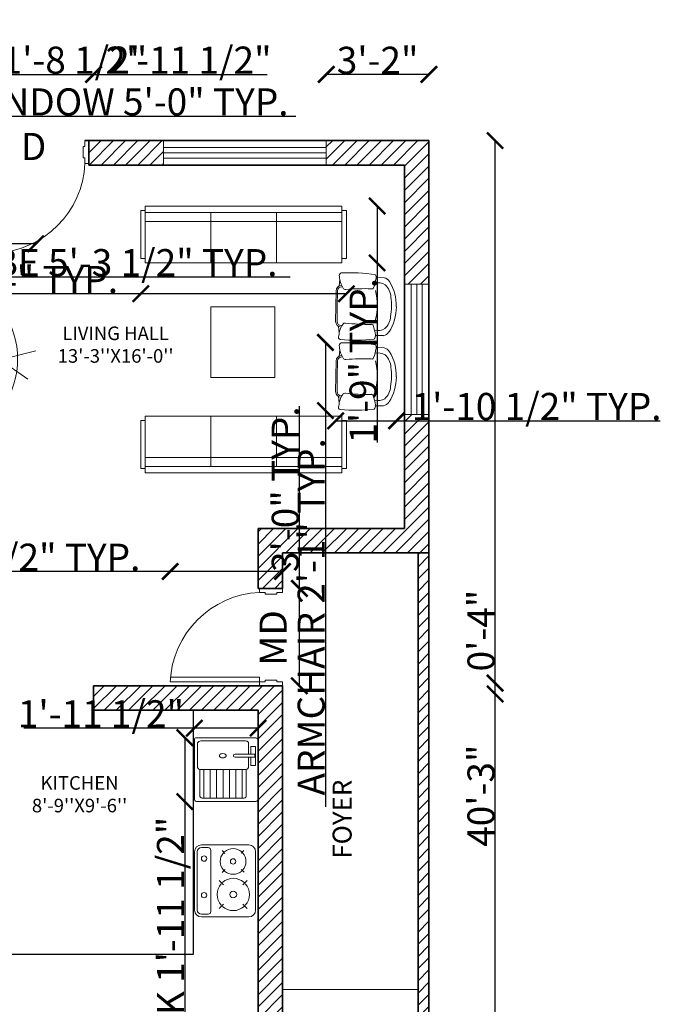
# Model space of a CAD drawing. Units: inches. Extents: x 1957 to 2456, y 1504 to 2088.
# Tile 6 of 6: x 2220 to 2456, y 1703 to 2066. Entities that reach past the tile are written whole.
import ezdxf

# ---------------------------------------------------------------- set-up
doc = ezdxf.new("R2010")
doc.units = ezdxf.units.IN
doc.header["$LTSCALE"] = 2
for name, color, linetype, lineweight in [('A-ANNO-DIMS', 2, 'Continuous', 18), ('A-ANNO-TEXT', 7, 'Continuous', 18), ('A-AREA-IDEN', 7, 'Continuous', 18), ('A-EQPM', 8, 'Continuous', 18), ('A-FLOR-FIXT', 8, 'Continuous', 18), ('A-FURN', 8, 'Continuous', 18), ('A-WALL-PATT', 8, 'Continuous', 13), ('Doors', 42, 'Continuous', 18), ('Kitchen', 60, 'Continuous', 25), ('Steps', 50, 'Continuous', 18), ('Walls', 7, 'Continuous', 35), ('Windows', 140, 'Continuous', 18)]:
    doc.layers.add(name, color=color, linetype=linetype, lineweight=lineweight)
doc.styles.get("Standard").update_dxf_attribs({"font": 'arial.ttf'})
doc.dimstyles.get("Standard").update_dxf_attribs({"dimtxt": 10, "dimasz": 6, "dimexe": 0.18, "dimexo": 0.0625, "dimgap": 0.09, "dimtad": 1, "dimdec": 1, "dimzin": 0, "dimdsep": 46, "dimlunit": 4, "dimtxsty": 'Standard', "dimblk": 'ARCHTICK', "dimcen": 0.09, "dimse1": 1, "dimse2": 1, "dimadec": 0, "dimazin": 0, "dimtfac": 1, "dimtdec": 1, "dimtofl": 0, "dimtmove": 0, "dimatfit": 3, "dimfxl": 1, "dimtolj": 1, "dimtzin": 0, "dimarcsym": 0})

# ---------------------------------------------------------------- blocks, each defined once
blk = doc.blocks.new('S_SINK12')
for p, q in [((0.25, 0.45), (0.25, 0)), ((0.35, 0.45), (0.35, 0)), ((0.45, 0.45), (0.45, 0)), ((0.55, 0.45), (0.55, 0)), ((0.65, 0.45), (0.65, 0)), ((0.75, 0.45), (0.75, 0)), ((0.85, 0.45), (0.85, 0))]:
    blk.add_line(p, q)
for points in [[(0, -0.469), (0, 0.469, -0.310961), (0.05, 0.5), (0.95, 0.5, -0.310466), (1, 0.469), (1, -0.469, -0.414214), (0.969, -0.5), (0.05, -0.5, -0.309971)], [(0.052, -0.195), (0.052, -0.242), (0.362, -0.242, 1), (0.362, -0.195)], [(0.5, -0.217), (0.503, -0.229, 0.107136), (0.516, -0.241, 0.076468), (0.534, -0.249), (0.554, -0.251), (0.575, -0.248, 0.076468), (0.592, -0.241, 0.107136), (0.604, -0.229), (0.608, -0.217), (0.604, -0.205, 0.107136), (0.592, -0.193, 0.076468), (0.575, -0.186), (0.554, -0.183), (0.532, -0.186, 0.076468), (0.516, -0.193, 0.107136), (0.503, -0.205)]]:
    blk.add_lwpolyline(points, format="xyb", close=True)
for points in [[(0.185, -0.001), (0.185, 0.419, -0.310466), (0.235, 0.45), (0.862, 0.45, -0.310466), (0.912, 0.419), (0.912, 0, -0.310466)], [(0.15, -0.195), (0.15, -0.031, -0.310466), (0.2, 0), (0.9, 0, -0.310466), (0.95, -0.031), (0.95, -0.419, -0.310466), (0.9, -0.45), (0.2, -0.45), (0.18, -0.448, -0.071009), (0.165, -0.442, -0.106323), (0.153, -0.432), (0.15, -0.422), (0.151, -0.419)]]:
    blk.add_lwpolyline(points, format="xyb")
for points in [[(0.114, -0.242), (0.114, -0.364), (0.039, -0.364), (0.039, -0.064), (0.114, -0.064), (0.114, -0.195)], [(0.15, -0.419), (0.15, -0.242)]]:
    blk.add_lwpolyline(points)
blk = doc.blocks.new('12PCOU09')
at = {"color": 0, "linetype": 'ByBlock'}
for p, q in [((26, 15), (3, 15)), ((26, -15), (3, -15))]:
    blk.add_line(p, q, dxfattribs=at)
for points in [[(2, 45), (2, 47), (24, 47), (24, 45)], [(2, -47), (2, -45), (24, -45), (24, -47)]]:
    blk.add_lwpolyline(points, close=True, dxfattribs=at)
for points in [[(2, -45), (0, -45), (0, 45), (2, 45)], [(3, -45), (3, 45)], [(7, 45), (7, -45)], [(24, 45), (26, 45), (26, -45), (24, -45)]]:
    blk.add_lwpolyline(points, dxfattribs=at)
blk = doc.blocks.new('banghe81')
for p, q in [((-500, 3000), (0, 3000)), ((-500, 2312), (-500, 3000)), ((0, 3000), (0, 0)), ((-925, 1843), (-450, 1517)), ((-607, 1930), (-419, 1930)), ((-607, 1117), (-607, 1930)), ((-419, 1930), (-419, 1117)), ((-107, 1742), (-419, 1867)), ((-107, 1305), (-107, 1742)), ((-450, 1517), (-1057, 1361)), ((-482, 1617), (-482, 1430)), ((-419, 1617), (-482, 1617)), ((-482, 1430), (-419, 1430)), ((-419, 1180), (-107, 1305)), ((-419, 1117), (-607, 1117)), ((-500, 0), (-500, 688)), ((0, 0), (-500, 0)), ((-500, 0), (-500, 0))]:
    blk.add_line(p, q)
blk.add_arc((695, 1500), 1445, 145.7945, 214.2055)
blk = doc.blocks.new('A$C198557BC')
for p, q in [((-0.412, 0.581), (-0.41, 0.695)), ((0.425, 0.571), (0.425, 0.685)), ((-0.291, 0.046), (-0.382, 0.055)), ((-0.299, 0.083), (-0.299, 0.085)), ((0, 0.02), (-0.22, 0.023)), ((0, 0), (-0.22, 0.003)), ((0, 0.02), (0.221, 0.017)), ((0, 0), (0.22, -0.003)), ((0.291, 0.039), (0.383, 0.046)), ((0.301, 0.077), (0.301, 0.078))]:
    blk.add_line(p, q)
for centre, radius, start, end in [((-0.003, 0.196), 0.675, 88.9141, 121.2698), ((0.005, 0.189), 0.683, 57.6049, 89.6023), ((-0.288, 0.668), 0.124, 121.5636, 167.5307), ((-0.132, 0.606), 0.205, 148.9368, 191.7767), ((-0.109, 0.514), 0.28, 94.1154, 135.1368), ((-0.012, 0.135), 0.669, 87.9714, 100.088), ((-0.041, -0.271), 1.076, 79.8996, 87.1923), ((0.131, 0.526), 0.263, 42.8435, 86.2186), ((0.304, 0.661), 0.124, 11.1649, 57.132), ((1.987, 0.194), 2.469, 171.2505, 182.7738), ((-0.42, 0.533), 0.0491, 69.3538, 131.4415), ((-0.498, -0.067), 0.653, 68.9876, 81.6584), ((-0.015, -0.198), 0.795, 73.9397, 105.2329), ((0.496, -0.078), 0.653, 97.0372, 109.708), ((0.146, 0.603), 0.205, 346.9189, 29.7588), ((0.427, 0.504), 0.0668, 46.1176, 99.1612), ((-0.269, 0.522), 0.0208, 332.4461, 75.1743), ((3.087, 0.412), 3.339, 178.2785, 184.601), ((-3.076, 0.483), 3.339, 354.0946, 0.4171), ((0.281, 0.516), 0.0208, 103.5213, 206.2495), ((-1.903, 0.273), 2.393, 354.9918, 6.6966), ((-0.281, 0.139), 0.0403, 300.8178, 7.8066), ((-0.444, 0.084), 0.0362, 194.4565, 300.6699), ((-0.452, 0.425), 0.374, 274.1336, 300.8386), ((-0.219, 0.083), 0.08, 179.3478, 269.3478), ((-0.219, 0.083), 0.06, 179.3478, 269.3478), ((0.221, 0.077), 0.08, 269.3478, 359.3478), ((0.221, 0.077), 0.06, 269.3478, 359.3478), ((0.284, 0.133), 0.0403, 170.889, 237.8778), ((0.462, 0.415), 0.374, 237.857, 264.562), ((0.446, 0.074), 0.0362, 238.0257, 344.2391)]:
    blk.add_arc(centre, radius, start, end)
blk = doc.blocks.new('AP0B05')
for p, q in [((35, 100), (35, 880)), ((75, 100), (75, 878.9))]:
    blk.add_line(p, q)
for points in [[(0, 100), (0, -100), (35, -100), (35, -50), (50, -50), (50, 50), (35, 50), (35, 100)], [(850, 100), (850, -100), (815, -100), (815, -50), (800, -50), (800, 50), (815, 50), (815, 100)]]:
    blk.add_lwpolyline(points, close=True)
blk.add_lwpolyline([(35, 100), (75, 100)])
blk.add_arc((-2.4, 62.6), 818.3, 2.62122, 87.37878)
blk = doc.blocks.new('WIN-48IN')
for p, q in [((0, 6.5), (48, 6.5)), ((0, 4.5), (48, 4.5)), ((0, 2.5), (48, 2.5))]:
    blk.add_line(p, q)
blk.add_lwpolyline([(0, 9), (48, 9), (48, 0), (0, 0)], close=True)
blk = doc.blocks.new('WIN-60IN')
for p, q in [((0, 6.5), (60, 6.5)), ((0, 4.5), (60, 4.5)), ((0, 2.5), (60, 2.5))]:
    blk.add_line(p, q)
blk.add_lwpolyline([(0, 9), (60, 9), (60, 0), (0, 0)], close=True)
blk = doc.blocks.new('_ArchTick')
at = {"color": 0, "linetype": 'ByBlock', "const_width": 0.15}
blk.add_lwpolyline([(-0.5, -0.5), (0.5, 0.5)], dxfattribs=at)
blk = doc.blocks.new('*D19')
at = {"layer": 'A-ANNO-DIMS', "color": 0, "lineweight": -2, "transparency": 16777216}
for p, q in [((2275.61, 1862.36), (2088.68, 1862.36)), ((2317.03, 1862.36), (2275.61, 1862.36))]:
    blk.add_line(p, q, dxfattribs=at)
at = {"layer": 'Defpoints', "color": 0, "transparency": 16777216}
for p in [(2275.61, 1862.36), (2275.61, 1856.15), (2317.03, 1856.15)]:
    blk.add_point(p, dxfattribs=at)
at = {"layer": 'A-ANNO-DIMS', "color": 0, "lineweight": -2, "transparency": 16777216, "xscale": 6, "yscale": 6, "zscale": 6, "rotation": 180}
blk.add_blockref('_ArchTick', (2275.61, 1862.36), dxfattribs=at)
at = {"layer": 'A-ANNO-DIMS', "color": 0, "lineweight": -2, "transparency": 16777216, "xscale": 6, "yscale": 6, "zscale": 6}
blk.add_blockref('_ArchTick', (2317.03, 1862.36), dxfattribs=at)
at = {"layer": 'A-ANNO-DIMS', "color": 0, "transparency": 16777216, "insert": (2179.14, 1867.63), "char_height": 10, "attachment_point": 5}
blk.add_mtext('\\A1;ENTRY DOOR 3\'-5 1/2" TYP.', dxfattribs=at)
blk = doc.blocks.new('*D20')
at = {"layer": 'A-ANNO-DIMS', "color": 0, "lineweight": -2, "transparency": 16777216}
for p, q in [((2323.25, 1856.15), (2323.25, 1923.28)), ((2323.25, 1820.22), (2323.25, 1856.15))]:
    blk.add_line(p, q, dxfattribs=at)
at = {"layer": 'Defpoints', "color": 0, "transparency": 16777216}
for p in [(2317.03, 1856.15), (2323.25, 1856.15), (2317.03, 1820.22)]:
    blk.add_point(p, dxfattribs=at)
at = {"layer": 'A-ANNO-DIMS', "color": 0, "lineweight": -2, "transparency": 16777216, "xscale": 6, "yscale": 6, "zscale": 6}
for p, rotation in [((2323.25, 1856.15), 90), ((2323.25, 1820.22), 270)]:
    blk.add_blockref('_ArchTick', p, dxfattribs=dict(at, rotation=rotation))
at = {"layer": 'A-ANNO-DIMS', "color": 0, "transparency": 16777216, "insert": (2318.05, 1892.71), "char_height": 10, "attachment_point": 5, "rotation": 90}
blk.add_mtext('\\A1;3\'-0" TYP.', dxfattribs=at)
blk = doc.blocks.new('*D25')
at = {"layer": 'A-ANNO-DIMS', "color": 0, "lineweight": -2, "transparency": 16777216}
for p, q in [((2129.18, 2030.22), (2189.18, 2030.22)), ((2189.18, 2030.22), (2321.9, 2030.22))]:
    blk.add_line(p, q, dxfattribs=at)
at = {"layer": 'Defpoints', "color": 0, "transparency": 16777216}
for p in [(2189.18, 2030.22), (2129.18, 2021.22), (2189.18, 2021.22)]:
    blk.add_point(p, dxfattribs=at)
at = {"layer": 'A-ANNO-DIMS', "color": 0, "lineweight": -2, "transparency": 16777216, "xscale": 6, "yscale": 6, "zscale": 6, "rotation": 180}
blk.add_blockref('_ArchTick', (2129.18, 2030.22), dxfattribs=at)
at = {"layer": 'A-ANNO-DIMS', "color": 0, "lineweight": -2, "transparency": 16777216, "xscale": 6, "yscale": 6, "zscale": 6}
blk.add_blockref('_ArchTick', (2189.18, 2030.22), dxfattribs=at)
at = {"layer": 'A-ANNO-DIMS', "color": 0, "transparency": 16777216, "insert": (2258.54, 2035.48), "char_height": 10, "attachment_point": 5}
blk.add_mtext('\\A1;WINDOW 5\'-0" TYP.', dxfattribs=at)
blk = doc.blocks.new('*D31')
at = {"layer": 'A-ANNO-DIMS', "color": 0, "lineweight": -2, "transparency": 16777216}
for p, q in [((2079.36, 1970.96), (2142.81, 1970.96)), ((2142.81, 1970.96), (2319.81, 1970.96))]:
    blk.add_line(p, q, dxfattribs=at)
at = {"layer": 'Defpoints', "color": 0, "transparency": 16777216}
for p in [(2079.36, 1980.47), (2142.81, 1980.47), (2142.81, 1970.96)]:
    blk.add_point(p, dxfattribs=at)
at = {"layer": 'A-ANNO-DIMS', "color": 0, "lineweight": -2, "transparency": 16777216, "xscale": 6, "yscale": 6, "zscale": 6, "rotation": 180}
blk.add_blockref('_ArchTick', (2079.36, 1970.96), dxfattribs=at)
at = {"layer": 'A-ANNO-DIMS', "color": 0, "lineweight": -2, "transparency": 16777216, "xscale": 6, "yscale": 6, "zscale": 6}
blk.add_blockref('_ArchTick', (2142.81, 1970.96), dxfattribs=at)
at = {"layer": 'A-ANNO-DIMS', "color": 0, "transparency": 16777216, "insert": (2234.31, 1976.22), "char_height": 10, "attachment_point": 5}
blk.add_mtext('\\A1;WARDROBE 5\'-3 1/2" TYP.', dxfattribs=at)
blk = doc.blocks.new('*D35')
at = {"layer": 'A-ANNO-DIMS', "color": 0, "lineweight": -2, "transparency": 16777216}
for p, q in [((2264.8, 1964.77), (2155.8, 1964.77)), ((2340.57, 1964.77), (2264.8, 1964.77))]:
    blk.add_line(p, q, dxfattribs=at)
at = {"layer": 'Defpoints', "color": 0, "transparency": 16777216}
for p in [(2264.8, 1976.14), (2340.57, 1976.14), (2264.8, 1964.77)]:
    blk.add_point(p, dxfattribs=at)
at = {"layer": 'A-ANNO-DIMS', "color": 0, "lineweight": -2, "transparency": 16777216, "xscale": 6, "yscale": 6, "zscale": 6, "rotation": 180}
blk.add_blockref('_ArchTick', (2264.8, 1964.77), dxfattribs=at)
at = {"layer": 'A-ANNO-DIMS', "color": 0, "lineweight": -2, "transparency": 16777216, "xscale": 6, "yscale": 6, "zscale": 6}
blk.add_blockref('_ArchTick', (2340.57, 1964.77), dxfattribs=at)
at = {"layer": 'A-ANNO-DIMS', "color": 0, "transparency": 16777216, "insert": (2207.3, 1970.03), "char_height": 10, "attachment_point": 5}
blk.add_mtext('\\A1;SOFA 6\'-4" TYP.', dxfattribs=at)
blk = doc.blocks.new('*D36')
at = {"layer": 'A-ANNO-DIMS', "color": 0, "lineweight": -2, "transparency": 16777216}
for p, q in [((2351.93, 1997.09), (2351.93, 1976.14)), ((2351.93, 1976.14), (2351.93, 1909.94))]:
    blk.add_line(p, q, dxfattribs=at)
at = {"layer": 'Defpoints', "color": 0, "transparency": 16777216}
for p in [(2340.57, 1997.09), (2340.57, 1976.14), (2351.93, 1976.14)]:
    blk.add_point(p, dxfattribs=at)
at = {"layer": 'A-ANNO-DIMS', "color": 0, "lineweight": -2, "transparency": 16777216, "xscale": 6, "yscale": 6, "zscale": 6}
for p, rotation in [((2351.93, 1997.09), 90), ((2351.93, 1976.14), 270)]:
    blk.add_blockref('_ArchTick', p, dxfattribs=dict(at, rotation=rotation))
at = {"layer": 'A-ANNO-DIMS', "color": 0, "transparency": 16777216, "insert": (2346.74, 1940.04), "char_height": 10, "attachment_point": 5, "rotation": 90}
blk.add_mtext('\\A1;1\'-9" TYP.', dxfattribs=at)
blk = doc.blocks.new('*D37')
at = {"layer": 'A-ANNO-DIMS', "color": 0, "lineweight": -2, "transparency": 16777216}
for p, q in [((2332.87, 1946.81), (2332.87, 1921.7)), ((2332.87, 1921.7), (2332.87, 1775.6))]:
    blk.add_line(p, q, dxfattribs=at)
at = {"layer": 'Defpoints', "color": 0, "transparency": 16777216}
for p in [(2336.64, 1946.81), (2332.87, 1921.7), (2336.64, 1921.7)]:
    blk.add_point(p, dxfattribs=at)
at = {"layer": 'A-ANNO-DIMS', "color": 0, "lineweight": -2, "transparency": 16777216, "xscale": 6, "yscale": 6, "zscale": 6}
for p, rotation in [((2332.87, 1946.81), 90), ((2332.87, 1921.7), 270)]:
    blk.add_blockref('_ArchTick', p, dxfattribs=dict(at, rotation=rotation))
at = {"layer": 'A-ANNO-DIMS', "color": 0, "transparency": 16777216, "insert": (2327.61, 1845.65), "char_height": 10, "attachment_point": 5, "rotation": 90}
blk.add_mtext('\\A1;ARMCHAIR 2\'-1" TYP.', dxfattribs=at)
blk = doc.blocks.new('*D38')
at = {"layer": 'A-ANNO-DIMS', "color": 0, "lineweight": -2, "transparency": 16777216}
for p, q in [((2336.64, 1917.93), (2359.07, 1917.93)), ((2359.07, 1917.93), (2456.34, 1917.93))]:
    blk.add_line(p, q, dxfattribs=at)
at = {"layer": 'Defpoints', "color": 0, "transparency": 16777216}
for p in [(2336.64, 1921.7), (2359.07, 1921.7), (2359.07, 1917.93)]:
    blk.add_point(p, dxfattribs=at)
at = {"layer": 'A-ANNO-DIMS', "color": 0, "lineweight": -2, "transparency": 16777216, "xscale": 6, "yscale": 6, "zscale": 6, "rotation": 180}
blk.add_blockref('_ArchTick', (2336.64, 1917.93), dxfattribs=at)
at = {"layer": 'A-ANNO-DIMS', "color": 0, "lineweight": -2, "transparency": 16777216, "xscale": 6, "yscale": 6, "zscale": 6}
blk.add_blockref('_ArchTick', (2359.07, 1917.93), dxfattribs=at)
at = {"layer": 'A-ANNO-DIMS', "color": 0, "transparency": 16777216, "insert": (2410.71, 1923.2), "char_height": 10, "attachment_point": 5}
blk.add_mtext('\\A1;1\'-10 1/2" TYP.', dxfattribs=at)
blk = doc.blocks.new('*D40')
at = {"layer": 'A-ANNO-DIMS', "color": 0, "lineweight": -2, "transparency": 16777216}
for p, q in [((2203.03, 1983.16), (2163.44, 1983.16)), ((2226.04, 1983.16), (2203.03, 1983.16))]:
    blk.add_line(p, q, dxfattribs=at)
at = {"layer": 'Defpoints', "color": 0, "transparency": 16777216}
for p in [(2203.03, 1983.16), (2203.03, 1973.36), (2226.04, 1973.36)]:
    blk.add_point(p, dxfattribs=at)
at = {"layer": 'A-ANNO-DIMS', "color": 0, "lineweight": -2, "transparency": 16777216, "xscale": 6, "yscale": 6, "zscale": 6, "rotation": 180}
blk.add_blockref('_ArchTick', (2203.03, 1983.16), dxfattribs=at)
at = {"layer": 'A-ANNO-DIMS', "color": 0, "lineweight": -2, "transparency": 16777216, "xscale": 6, "yscale": 6, "zscale": 6}
blk.add_blockref('_ArchTick', (2226.04, 1983.16), dxfattribs=at)
at = {"layer": 'A-ANNO-DIMS', "color": 0, "transparency": 16777216, "insert": (2180.24, 1988.27), "char_height": 10, "attachment_point": 5}
blk.add_mtext('\\A1;1\'-11"', dxfattribs=at)
blk = doc.blocks.new('*D41')
at = {"layer": 'A-ANNO-DIMS', "color": 0, "lineweight": -2, "transparency": 16777216}
for p, q in [((2281, 1801.1), (2281, 1777.56)), ((2281, 1777.56), (2281, 1677.29))]:
    blk.add_line(p, q, dxfattribs=at)
at = {"layer": 'Defpoints', "color": 0, "transparency": 16777216}
for p in [(2284.53, 1801.1), (2281, 1777.56), (2284.53, 1777.56)]:
    blk.add_point(p, dxfattribs=at)
at = {"layer": 'A-ANNO-DIMS', "color": 0, "lineweight": -2, "transparency": 16777216, "xscale": 6, "yscale": 6, "zscale": 6}
for p, rotation in [((2281, 1801.1), 90), ((2281, 1777.56), 270)]:
    blk.add_blockref('_ArchTick', p, dxfattribs=dict(at, rotation=rotation))
at = {"layer": 'A-ANNO-DIMS', "color": 0, "transparency": 16777216, "insert": (2275.74, 1724.42), "char_height": 10, "attachment_point": 5, "rotation": 90}
blk.add_mtext('\\A1;SINK 1\'-11 1/2"', dxfattribs=at)
blk = doc.blocks.new('*D42')
at = {"layer": 'A-ANNO-DIMS', "color": 0, "lineweight": -2, "transparency": 16777216}
for p, q in [((2284.53, 1804.64), (2221.64, 1804.64)), ((2308.03, 1804.64), (2284.53, 1804.64))]:
    blk.add_line(p, q, dxfattribs=at)
at = {"layer": 'Defpoints', "color": 0, "transparency": 16777216}
for p in [(2284.53, 1804.64), (2284.53, 1801.1), (2308.03, 1801.1)]:
    blk.add_point(p, dxfattribs=at)
at = {"layer": 'A-ANNO-DIMS', "color": 0, "lineweight": -2, "transparency": 16777216, "xscale": 6, "yscale": 6, "zscale": 6, "rotation": 180}
blk.add_blockref('_ArchTick', (2284.53, 1804.64), dxfattribs=at)
at = {"layer": 'A-ANNO-DIMS', "color": 0, "lineweight": -2, "transparency": 16777216, "xscale": 6, "yscale": 6, "zscale": 6}
blk.add_blockref('_ArchTick', (2308.03, 1804.64), dxfattribs=at)
at = {"layer": 'A-ANNO-DIMS', "color": 0, "transparency": 16777216, "insert": (2250.09, 1809.9), "char_height": 10, "attachment_point": 5}
blk.add_mtext('\\A1;1\'-11 1/2"', dxfattribs=at)
blk = doc.blocks.new('*D46')
at = {"layer": 'A-ANNO-DIMS', "color": 0, "lineweight": -2, "transparency": 16777216}
blk.add_line((2395.43, 1538.22), (2395.43, 2021.22), dxfattribs=at)
at = {"layer": 'Defpoints', "color": 0, "transparency": 16777216}
for p in [(2371.03, 2021.22), (2395.43, 2021.22), (2371.03, 1538.22)]:
    blk.add_point(p, dxfattribs=at)
at = {"layer": 'A-ANNO-DIMS', "color": 0, "lineweight": -2, "transparency": 16777216, "xscale": 6, "yscale": 6, "zscale": 6}
for p, rotation in [((2395.43, 2021.22), 90), ((2395.43, 1538.22), 270)]:
    blk.add_blockref('_ArchTick', p, dxfattribs=dict(at, rotation=rotation))
at = {"layer": 'A-ANNO-DIMS', "color": 0, "transparency": 16777216, "insert": (2390.23, 1779.72), "char_height": 10, "attachment_point": 5, "rotation": 90}
blk.add_mtext('\\A1;40\'-3"', dxfattribs=at)
blk = doc.blocks.new('*D48')
at = {"layer": 'A-ANNO-DIMS', "color": 0, "lineweight": -2, "transparency": 16777216}
for p, q in [((2189.18, 2045.62), (2209.75, 2045.62)), ((2209.75, 2045.62), (2264.87, 2045.62))]:
    blk.add_line(p, q, dxfattribs=at)
at = {"layer": 'Defpoints', "color": 0, "transparency": 16777216}
for p in [(2209.75, 2045.62), (2189.18, 2021.22), (2209.75, 2021.22)]:
    blk.add_point(p, dxfattribs=at)
at = {"layer": 'A-ANNO-DIMS', "color": 0, "lineweight": -2, "transparency": 16777216, "xscale": 6, "yscale": 6, "zscale": 6, "rotation": 180}
blk.add_blockref('_ArchTick', (2189.18, 2045.62), dxfattribs=at)
at = {"layer": 'A-ANNO-DIMS', "color": 0, "lineweight": -2, "transparency": 16777216, "xscale": 6, "yscale": 6, "zscale": 6}
blk.add_blockref('_ArchTick', (2209.75, 2045.62), dxfattribs=at)
at = {"layer": 'A-ANNO-DIMS', "color": 0, "transparency": 16777216, "insert": (2240.31, 2050.88), "char_height": 10, "attachment_point": 5}
blk.add_mtext('\\A1;1\'-8 1/2"', dxfattribs=at)
blk = doc.blocks.new('*D49')
at = {"layer": 'A-ANNO-DIMS', "color": 0, "lineweight": -2, "transparency": 16777216}
blk.add_line((2371.03, 2045.62), (2333.18, 2045.62), dxfattribs=at)
at = {"layer": 'Defpoints', "color": 0, "transparency": 16777216}
for p in [(2333.18, 2045.62), (2333.18, 2021.22), (2371.03, 2021.22)]:
    blk.add_point(p, dxfattribs=at)
at = {"layer": 'A-ANNO-DIMS', "color": 0, "lineweight": -2, "transparency": 16777216, "xscale": 6, "yscale": 6, "zscale": 6, "rotation": 180}
blk.add_blockref('_ArchTick', (2333.18, 2045.62), dxfattribs=at)
at = {"layer": 'A-ANNO-DIMS', "color": 0, "lineweight": -2, "transparency": 16777216, "xscale": 6, "yscale": 6, "zscale": 6}
blk.add_blockref('_ArchTick', (2371.03, 2045.62), dxfattribs=at)
at = {"layer": 'A-ANNO-DIMS', "color": 0, "transparency": 16777216, "insert": (2352.11, 2050.82), "char_height": 10, "attachment_point": 5}
blk.add_mtext('\\A1;3\'-2"', dxfattribs=at)
blk = doc.blocks.new('*D50')
at = {"layer": 'A-ANNO-DIMS', "color": 0, "lineweight": -2, "transparency": 16777216}
blk.add_line((2040.63, 2012.22), (2040.63, 1968.25), dxfattribs=at)
at = {"layer": 'Defpoints', "color": 0, "transparency": 16777216}
for p in [(2362.03, 2012.22), (2040.63, 1968.25), (2362.03, 1968.25)]:
    blk.add_point(p, dxfattribs=at)
at = {"layer": 'A-ANNO-DIMS', "color": 0, "lineweight": -2, "transparency": 16777216, "xscale": 6, "yscale": 6, "zscale": 6}
for p, rotation in [((2040.63, 2012.22), 90), ((2040.63, 1968.25), 270)]:
    blk.add_blockref('_ArchTick', p, dxfattribs=dict(at, rotation=rotation))
at = {"layer": 'A-ANNO-DIMS', "color": 0, "transparency": 16777216, "insert": (2035.43, 1990.23), "char_height": 10, "attachment_point": 5, "rotation": 90}
blk.add_mtext('\\A1;3\'-8"', dxfattribs=at)
blk = doc.blocks.new('*D56')
at = {"layer": 'A-ANNO-DIMS', "color": 0, "lineweight": -2, "transparency": 16777216}
blk.add_line((2040.63, 1688.22), (2040.63, 1869.22), dxfattribs=at)
at = {"layer": 'Defpoints', "color": 0, "transparency": 16777216}
for p in [(2040.63, 1869.22), (2367.03, 1869.22), (2367.03, 1688.22)]:
    blk.add_point(p, dxfattribs=at)
at = {"layer": 'A-ANNO-DIMS', "color": 0, "lineweight": -2, "transparency": 16777216, "xscale": 6, "yscale": 6, "zscale": 6}
for p, rotation in [((2040.63, 1869.22), 90), ((2040.63, 1688.22), 270)]:
    blk.add_blockref('_ArchTick', p, dxfattribs=dict(at, rotation=rotation))
at = {"layer": 'A-ANNO-DIMS', "color": 0, "transparency": 16777216, "insert": (2035.44, 1778.72), "char_height": 10, "attachment_point": 5, "rotation": 90}
blk.add_mtext('\\A1;15\'-1"', dxfattribs=at)
blk = doc.blocks.new('*D61')
at = {"layer": 'A-ANNO-DIMS', "color": 0, "lineweight": -2, "transparency": 16777216}
for p, q in [((2211.8, 2045.62), (2247.38, 2045.62)), ((2247.38, 2045.62), (2311.38, 2045.62))]:
    blk.add_line(p, q, dxfattribs=at)
at = {"layer": 'Defpoints', "color": 0, "transparency": 16777216}
for p in [(2247.38, 2045.62), (2211.8, 1820.22), (2247.38, 1820.22)]:
    blk.add_point(p, dxfattribs=at)
at = {"layer": 'A-ANNO-DIMS', "color": 0, "lineweight": -2, "transparency": 16777216, "xscale": 6, "yscale": 6, "zscale": 6, "rotation": 180}
blk.add_blockref('_ArchTick', (2211.8, 2045.62), dxfattribs=at)
at = {"layer": 'A-ANNO-DIMS', "color": 0, "lineweight": -2, "transparency": 16777216, "xscale": 6, "yscale": 6, "zscale": 6}
blk.add_blockref('_ArchTick', (2247.38, 2045.62), dxfattribs=at)
at = {"layer": 'A-ANNO-DIMS', "color": 0, "transparency": 16777216, "insert": (2282.38, 2050.88), "char_height": 10, "attachment_point": 5}
blk.add_mtext('\\A1;2\'-11 1/2"', dxfattribs=at)
blk = doc.blocks.new('*D64')
at = {"layer": 'A-ANNO-DIMS', "color": 0, "lineweight": -2, "transparency": 16777216}
for p, q in [((2290.6, 1513.82), (2314.26, 1513.82)), ((2314.26, 1513.82), (2377.15, 1513.82))]:
    blk.add_line(p, q, dxfattribs=at)
at = {"layer": 'Defpoints', "color": 0, "transparency": 16777216}
for p in [(2290.6, 1933.88), (2314.26, 1933.88), (2314.26, 1513.82)]:
    blk.add_point(p, dxfattribs=at)
at = {"layer": 'A-ANNO-DIMS', "color": 0, "lineweight": -2, "transparency": 16777216, "xscale": 6, "yscale": 6, "zscale": 6, "rotation": 180}
blk.add_blockref('_ArchTick', (2290.6, 1513.82), dxfattribs=at)
at = {"layer": 'A-ANNO-DIMS', "color": 0, "lineweight": -2, "transparency": 16777216, "xscale": 6, "yscale": 6, "zscale": 6}
blk.add_blockref('_ArchTick', (2314.26, 1513.82), dxfattribs=at)
at = {"layer": 'A-ANNO-DIMS', "color": 0, "transparency": 16777216, "insert": (2348.71, 1519.08), "char_height": 10, "attachment_point": 5}
blk.add_mtext('\\A1;1\'-11 1/2"', dxfattribs=at)
blk = doc.blocks.new('*D65')
at = {"layer": 'A-ANNO-DIMS', "color": 0, "lineweight": -2, "transparency": 16777216}
for p, q in [((2040.63, 1959.92), (2040.63, 1992.85)), ((2040.63, 1933.88), (2040.63, 1959.92))]:
    blk.add_line(p, q, dxfattribs=at)
at = {"layer": 'Defpoints', "color": 0, "transparency": 16777216}
for p in [(2040.63, 1959.92), (2290.6, 1959.92), (2290.6, 1933.88)]:
    blk.add_point(p, dxfattribs=at)
at = {"layer": 'A-ANNO-DIMS', "color": 0, "lineweight": -2, "transparency": 16777216, "xscale": 6, "yscale": 6, "zscale": 6}
for p, rotation in [((2040.63, 1959.92), 90), ((2040.63, 1933.88), 270)]:
    blk.add_blockref('_ArchTick', p, dxfattribs=dict(at, rotation=rotation))
at = {"layer": 'A-ANNO-DIMS', "color": 0, "transparency": 16777216, "insert": (2035.52, 1979.39), "char_height": 10, "attachment_point": 5, "rotation": 90}
blk.add_mtext('\\A1;2\'-2"', dxfattribs=at)
blk = doc.blocks.new('*D66')
at = {"layer": 'A-ANNO-DIMS', "color": 0, "lineweight": -2, "transparency": 16777216}
for p, q in [((2284.61, 1513.82), (2307.13, 1513.82)), ((2307.13, 1513.82), (2370.02, 1513.82))]:
    blk.add_line(p, q, dxfattribs=at)
at = {"layer": 'Defpoints', "color": 0, "transparency": 16777216}
for p in [(2284.61, 1737.54), (2307.13, 1737.54), (2307.13, 1513.82)]:
    blk.add_point(p, dxfattribs=at)
at = {"layer": 'A-ANNO-DIMS', "color": 0, "lineweight": -2, "transparency": 16777216, "xscale": 6, "yscale": 6, "zscale": 6, "rotation": 180}
blk.add_blockref('_ArchTick', (2284.61, 1513.82), dxfattribs=at)
at = {"layer": 'A-ANNO-DIMS', "color": 0, "lineweight": -2, "transparency": 16777216, "xscale": 6, "yscale": 6, "zscale": 6}
blk.add_blockref('_ArchTick', (2307.13, 1513.82), dxfattribs=at)
at = {"layer": 'A-ANNO-DIMS', "color": 0, "transparency": 16777216, "insert": (2341.58, 1519.08), "char_height": 10, "attachment_point": 5}
blk.add_mtext('\\A1;1\'-10 1/2"', dxfattribs=at)
blk = doc.blocks.new('*D67')
at = {"layer": 'A-ANNO-DIMS', "color": 0, "lineweight": -2, "transparency": 16777216}
for p, q in [((2040.63, 1761.57), (2040.63, 1817.8)), ((2040.63, 1735.04), (2040.63, 1761.57))]:
    blk.add_line(p, q, dxfattribs=at)
at = {"layer": 'Defpoints', "color": 0, "transparency": 16777216}
for p in [(2040.63, 1761.57), (2287.11, 1761.57), (2287.11, 1735.04)]:
    blk.add_point(p, dxfattribs=at)
at = {"layer": 'A-ANNO-DIMS', "color": 0, "lineweight": -2, "transparency": 16777216, "xscale": 6, "yscale": 6, "zscale": 6}
for p, rotation in [((2040.63, 1761.57), 90), ((2040.63, 1735.04), 270)]:
    blk.add_blockref('_ArchTick', p, dxfattribs=dict(at, rotation=rotation))
at = {"layer": 'A-ANNO-DIMS', "color": 0, "transparency": 16777216, "insert": (2035.37, 1792.69), "char_height": 10, "attachment_point": 5, "rotation": 90}
blk.add_mtext('\\A1;2\'-2 1/2"', dxfattribs=at)
blk = doc.blocks.new('*D68')
at = {"layer": 'A-ANNO-DIMS', "color": 0, "lineweight": -2, "transparency": 16777216}
for p, q in [((2395.43, 1821.22), (2395.43, 1853.98)), ((2395.43, 1817.22), (2395.43, 1821.22))]:
    blk.add_line(p, q, dxfattribs=at)
at = {"layer": 'Defpoints', "color": 0, "transparency": 16777216}
for p in [(2149.03, 1821.22), (2395.43, 1821.22), (2149.03, 1817.22)]:
    blk.add_point(p, dxfattribs=at)
at = {"layer": 'A-ANNO-DIMS', "color": 0, "lineweight": -2, "transparency": 16777216, "xscale": 6, "yscale": 6, "zscale": 6}
for p, rotation in [((2395.43, 1821.22), 90), ((2395.43, 1817.22), 270)]:
    blk.add_blockref('_ArchTick', p, dxfattribs=dict(at, rotation=rotation))
at = {"layer": 'A-ANNO-DIMS', "color": 0, "transparency": 16777216, "insert": (2390.24, 1840.6), "char_height": 10, "attachment_point": 5, "rotation": 90}
blk.add_mtext('\\A1;0\'-4"', dxfattribs=at)

msp = doc.modelspace()

# ---------------------------------------------------------------- hatches: boundary and pattern name
at = {"layer": 'A-WALL-PATT', "transparency": 33554585}
h = msp.add_hatch(dxfattribs=at)
h.set_pattern_fill('ANSI31', color=256)
h.paths.add_polyline_path([(2129.18, 2021.22), (2065.03, 2021.22), (2065.03, 1857.22), (2074.03, 1857.22), (2074.03, 1869.22), (2115.8, 1869.22), (2115.8, 1878.22), (2074.03, 1878.22), (2074.03, 2012.22), (2129.18, 2012.22)])
h.paths.add_polyline_path([(2209.75, 2021.22), (2189.18, 2021.22), (2189.18, 2012.22), (2194.03, 2012.22), (2194.03, 1878.22), (2190.56, 1878.22), (2190.56, 1869.22), (2203.03, 1869.22), (2203.03, 2012.22), (2209.75, 2012.22)])
h.paths.add_polyline_path([(2273.18, 2021.22), (2245.68, 2021.22), (2245.68, 2012.22), (2273.18, 2012.22)])
h.paths.add_polyline_path([(2371.03, 2021.22), (2333.18, 2021.22), (2333.18, 2012.22), (2362.03, 2012.22), (2362.03, 1968.25), (2371.03, 1968.25)])
h.paths.add_polyline_path([(2371.03, 1869.22), (2367.03, 1869.22), (2367.03, 1546.41), (2371.03, 1546.41)])
h.paths.add_polyline_path([(2317.03, 1820.22), (2247.38, 1820.22), (2247.38, 1811.22), (2308.03, 1811.22), (2308.03, 1697.22), (2284.03, 1697.22), (2284.03, 1688.22), (2317.03, 1688.22)])
h.paths.add_polyline_path([(2236.03, 1697.22), (2203.03, 1697.22), (2203.03, 1811.22), (2211.8, 1811.22), (2211.8, 1820.22), (2194.03, 1820.22), (2194.03, 1619.22), (2074.03, 1619.22), (2074.03, 1610.22), (2203.03, 1610.22), (2203.03, 1688.22), (2236.03, 1688.22)])
h.paths.add_polyline_path([(2153.03, 1869.22), (2155.49, 1869.22), (2155.49, 1877.47), (2155.49, 1878.22), (2146.03, 1878.22), (2146.03, 1871.1), (2146.03, 1869.22), (2149.03, 1869.22), (2149.03, 1821.22), (2074.03, 1821.22), (2074.03, 1833.22), (2065.03, 1833.22), (2065.03, 1805.22), (2074.03, 1805.22), (2074.03, 1817.22), (2149.03, 1817.22), (2149.03, 1769.22), (2146.03, 1769.22), (2146.03, 1760.22), (2153.03, 1760.22), (2156.02, 1760.22), (2156.02, 1760.87), (2156.02, 1769.11), (2153.03, 1769.11)])
h.paths.add_polyline_path([(2074.03, 1781.22), (2065.03, 1781.22), (2065.03, 1758.05), (2074.03, 1758.05), (2074.03, 1760.22), (2115.8, 1760.22), (2115.8, 1767.33), (2115.8, 1769.22), (2074.03, 1769.22)])
h = msp.add_hatch(dxfattribs=at)
h.set_pattern_fill('ANSI31', color=256)
h.paths.add_polyline_path([(2371.03, 1920.25), (2362.03, 1920.25), (2362.03, 1878.22), (2308.03, 1878.22), (2308.03, 1869.22), (2308.03, 1856.15), (2317.03, 1856.15), (2317.03, 1869.22), (2371.03, 1869.22)])
h.paths.add_polyline_path([(2074.03, 1710.05), (2065.03, 1710.05), (2065.03, 1538.22), (2203.03, 1538.22), (2220.79, 1538.22), (2220.79, 1547.22), (2203.03, 1547.22), (2074.03, 1547.22)])

# ---------------------------------------------------------------- linework, layer by layer
at = {"layer": 'A-EQPM'}
for p, q in [((2304.63, 1761.57), (2287.11, 1761.57)), ((2289.61, 1760.57), (2287.11, 1760.57)), ((2284.61, 1759.07), (2284.61, 1737.54)), ((2285.61, 1759.07), (2285.61, 1737.54)), ((2290.61, 1737.04), (2290.61, 1759.57)), ((2294.75, 1759.49), (2295.78, 1758.44)), ((2302.8, 1759.54), (2301.75, 1758.51)), ((2307.13, 1737.54), (2307.13, 1759.07)), ((2294.8, 1751.44), (2295.85, 1752.47)), ((2302.85, 1751.49), (2301.81, 1752.54)), ((2293.72, 1748.45), (2295.29, 1746.87)), ((2304.02, 1748.46), (2302.44, 1746.88)), ((2293.72, 1738.14), (2295.3, 1739.72)), ((2304.03, 1738.15), (2302.45, 1739.73)), ((2287.11, 1736.04), (2289.61, 1736.04)), ((2287.11, 1735.04), (2304.63, 1735.04))]:
    msp.add_line(p, q, dxfattribs=at)
for centre, radius in [((2288.11, 1756.56), 1), ((2298.8, 1755.49), 1), ((2288.11, 1743.05), 1), ((2298.87, 1743.3), 1.26)]:
    msp.add_circle(centre, radius, dxfattribs=at)
for centre, radius, start, end in [((2287.11, 1759.07), 2.5, 90, 180), ((2287.11, 1759.07), 1.5, 90, 180), ((2289.61, 1759.57), 1, 0, 90), ((2304.63, 1759.07), 2.5, 0, 90), ((2298.8, 1755.49), 4.76, 138.017, 221.983), ((2298.8, 1755.49), 4.76, 48.017, 131.983), ((2298.8, 1755.49), 4.76, 318.017, 41.983), ((2298.8, 1755.49), 4.76, 228.017, 311.983), ((2298.87, 1743.3), 5.96, 138.017, 221.983), ((2298.87, 1743.3), 5.96, 48.017, 131.983), ((2298.87, 1743.3), 5.96, 318.017, 41.983), ((2298.87, 1743.3), 5.96, 228.017, 311.983), ((2287.11, 1737.54), 2.5, 180, 270), ((2287.11, 1737.54), 1.5, 180, 270), ((2289.61, 1737.04), 1, 270, 0), ((2304.63, 1737.54), 2.5, 270, 0)]:
    msp.add_arc(centre, radius, start, end, dxfattribs=at)
at = {"layer": 'A-FURN'}
msp.add_lwpolyline([(2290.6, 1959.92), (2314.26, 1959.92), (2314.26, 1933.88), (2290.6, 1933.88)], close=True, dxfattribs=at)
at = {"layer": 'Kitchen'}
for p, q in [((2284.03, 1811.22), (2284.03, 1721.22)), ((2284.03, 1721.22), (2203.03, 1721.22))]:
    msp.add_line(p, q, dxfattribs=at)
at = {"layer": 'Steps'}
msp.add_line((2317.03, 1708.22), (2367.03, 1708.22), dxfattribs=at)
at = {"layer": 'Walls'}
for p, q in [((2371.03, 2021.22), (2244.2, 2021.22)), ((2245.68, 2021.22), (2245.68, 2012.22)), ((2371.03, 2021.22), (2371.03, 1538.22)), ((2362.03, 2012.22), (2245.68, 2012.22)), ((2362.03, 2012.22), (2362.03, 1878.22)), ((2362.03, 1878.22), (2308.03, 1878.22)), ((2308.03, 1878.22), (2308.03, 1869.22)), ((2308.03, 1856.15), (2308.03, 1869.22)), ((2371.03, 1869.22), (2317.03, 1869.22)), ((2317.03, 1856.15), (2317.03, 1869.22)), ((2367.03, 1869.22), (2367.03, 1546.41)), ((2317.03, 1856.15), (2308.03, 1856.15)), ((2247.38, 1820.22), (2247.38, 1811.22)), ((2317.03, 1820.22), (2247.38, 1820.22)), ((2317.03, 1820.22), (2317.03, 1688.22)), ((2308.03, 1811.22), (2247.38, 1811.22)), ((2308.03, 1811.22), (2308.03, 1697.22))]:
    msp.add_line(p, q, dxfattribs=at)

# ---------------------------------------------------------------- block references
at = {"layer": 'A-FLOR-FIXT', "xscale": 23.49981946469933, "yscale": 23.49981946469933, "zscale": 23.49981946469933, "rotation": 180}
msp.add_blockref('S_SINK12', (2308.03, 1789.33), dxfattribs=at)
at = {"layer": 'A-FURN'}
for name, p, xscale, yscale, zscale, rotation in [('12PCOU09', (2302.69, 1997.09), -0.8060007279000467, 0.8060007279000467, 0.8060007279000467, 90), ('banghe81', (2203.03, 1973.36), 0.0217636098217213, 0.0217636098217213, 0.0217636098217213, 180), ('A$C198557BC', (2336.71, 1960.19), 25.58518477870162, 25.58518477870162, 25.58518477870162, 270), ('A$C198557BC', (2336.71, 1934.35), 25.58518477870162, 25.58518477870162, 25.58518477870162, 270), ('12PCOU09', (2302.69, 1898.7), 0.8060007279000467, 0.8060007279000467, 0.8060007279000467, 90)]:
    msp.add_blockref(name, p, dxfattribs=dict(at, xscale=xscale, yscale=yscale, zscale=zscale, rotation=rotation))
at = {"layer": 'Doors', "yscale": 0.042270002124437, "zscale": 0.042270002124437}
for p, xscale, rotation in [((2209.75, 2016.99), -0.042270002124437, 180), ((2312.81, 1820.22), 0.042270002124437, 90)]:
    msp.add_blockref('AP0B05', p, dxfattribs=dict(at, xscale=xscale, rotation=rotation))
at = {"layer": 'Windows'}
msp.add_blockref('WIN-60IN', (2273.18, 2012.22), dxfattribs=at)
at = {"layer": 'Windows', "rotation": 89.9999999999985}
msp.add_blockref('WIN-48IN', (2371.03, 1920.25), dxfattribs=at)

# ---------------------------------------------------------------- texts
at = {"layer": 'A-ANNO-TEXT'}
msp.add_text('D', height=10, dxfattribs=at).set_placement((2220.55, 2014.04))
msp.add_text('MD', height=10, rotation=90, dxfattribs=at).set_placement((2318.57, 1827.65))
at = {"layer": 'A-AREA-IDEN', "char_height": 5, "attachment_point": 1}
for s, insert in [("\\pxqc;LIVING HALL\\P13'-3''X16'-0''", (2229.41, 1952.67)), ("\\pxqc;KITCHEN\\P8'-9''X9'-6''", (2216.12, 1786.92))]:
    msp.add_mtext_dynamic_manual_height_columns(s, width=52.1707, gutter_width=12.5, heights=[0], dxfattribs=dict(at, insert=insert))
at = {"layer": 'A-AREA-IDEN', "insert": (2335.52, 1744.97), "char_height": 7, "attachment_point": 1, "rotation": 90}
msp.add_mtext_dynamic_manual_height_columns('\\pxqc;FOYER', width=52.1707, gutter_width=12.5, heights=[0], dxfattribs=at)

# ---------------------------------------------------------------- dimensions: what is measured, and where the dimension line sits
at = {"layer": 'A-ANNO-DIMS'}
for base, p1, p2, picture, middle in [((2209.75, 2045.62), (2189.18, 2021.22), (2209.75, 2021.22), '*D48', (2240.31, 2050.88)), ((2247.38, 2045.62), (2211.8, 1820.22), (2247.38, 1820.22), '*D61', (2282.38, 2050.88)), ((2333.1785, 2045.6189), (2371.0339, 2021.2189), (2333.1785, 2021.2189), '*D49', (2352.1062, 2050.8181)), ((2314.26, 1513.82), (2290.6, 1933.88), (2314.26, 1933.88), '*D64', (2348.71, 1519.08)), ((2307.13, 1513.82), (2284.61, 1737.54), (2307.13, 1737.54), '*D66', (2341.58, 1519.08))]:
    dim = msp.add_linear_dim(base=base, p1=p1, p2=p2, dimstyle='Standard', override={"dimdec": 1, "dimlfac": 1, "dimrnd": 0, "dimzin": 1, "dimdsep": 46, "dimlunit": 4, "dimfrac": 2}, dxfattribs=at)
    dim.commit()
    dim.dimension.update_dxf_attribs({"geometry": picture, "text_midpoint": middle})
for base, p1, p2, text, picture, middle in [((2189.18, 2030.22), (2129.18, 2021.22), (2189.18, 2021.22), 'WINDOW <> TYP.', '*D25', (2258.54, 2035.48)), ((2142.8119, 1970.9563), (2079.3559, 1980.4747), (2142.8119, 1980.4747), 'WARDROBE <> TYP.', '*D31', (2234.3112, 1976.2236)), ((2359.07, 1917.93), (2336.64, 1921.7), (2359.07, 1921.7), '<> TYP.', '*D38', (2410.71, 1923.2))]:
    dim = msp.add_linear_dim(base=base, p1=p1, p2=p2, text=text, dimstyle='Standard', override={"dimdec": 1, "dimlfac": 1, "dimrnd": 0, "dimzin": 1, "dimdsep": 46, "dimlunit": 4, "dimfrac": 2}, dxfattribs=at)
    dim.commit()
    dim.dimension.update_dxf_attribs({"geometry": picture, "text_midpoint": middle})
for base, p1, p2, angle, picture, middle in [((2395.43, 2021.22), (2371.03, 1538.22), (2371.03, 2021.22), 90, '*D46', (2390.23, 1779.72)), ((2040.63, 1968.25), (2362.03, 2012.22), (2362.03, 1968.25), 90, '*D50', (2035.43, 1990.23)), ((2040.63, 1959.92), (2290.6, 1933.88), (2290.6, 1959.92), 90, '*D65', (2035.52, 1979.39)), ((2203.03, 1983.16), (2226.04, 1973.36), (2203.03, 1973.36), 180, '*D40', (2180.24, 1988.27)), ((2040.63, 1869.22), (2367.03, 1688.22), (2367.03, 1869.22), 90, '*D56', (2035.44, 1778.72)), ((2395.43, 1821.22), (2149.03, 1817.22), (2149.03, 1821.22), 90, '*D68', (2390.24, 1840.6)), ((2284.53, 1804.64), (2308.03, 1801.1), (2284.53, 1801.1), 180, '*D42', (2250.09, 1809.9)), ((2040.63, 1761.57), (2287.11, 1735.04), (2287.11, 1761.57), 90, '*D67', (2035.37, 1792.69))]:
    dim = msp.add_linear_dim(base=base, p1=p1, p2=p2, angle=angle, dimstyle='Standard', override={"dimdec": 1, "dimlfac": 1, "dimrnd": 0, "dimzin": 1, "dimdsep": 46, "dimlunit": 4, "dimfrac": 2}, dxfattribs=at)
    dim.commit()
    dim.dimension.update_dxf_attribs({"geometry": picture, "text_midpoint": middle})
for base, p1, p2, angle, text, picture, middle in [((2351.9319, 1976.1351), (2340.5673, 1997.0911), (2340.5673, 1976.1351), 270, '<> TYP.', '*D36', (2346.7361, 1940.0383)), ((2264.8, 1964.77), (2340.57, 1976.14), (2264.8, 1976.14), 180, 'SOFA <> TYP.', '*D35', (2207.3, 1970.03)), ((2332.87, 1921.7), (2336.64, 1946.81), (2336.64, 1921.7), 270, 'ARMCHAIR <> TYP.', '*D37', (2327.61, 1845.65)), ((2323.25, 1856.15), (2317.03, 1820.22), (2317.03, 1856.15), 90, '<> TYP.', '*D20', (2318.05, 1892.71)), ((2275.61, 1862.36), (2317.03, 1856.15), (2275.61, 1856.15), 180, 'ENTRY DOOR <> TYP.', '*D19', (2179.14, 1867.63)), ((2281, 1777.56), (2284.53, 1801.1), (2284.53, 1777.56), 270, 'SINK <>', '*D41', (2275.74, 1724.42))]:
    dim = msp.add_linear_dim(base=base, p1=p1, p2=p2, angle=angle, text=text, dimstyle='Standard', override={"dimdec": 1, "dimlfac": 1, "dimrnd": 0, "dimzin": 1, "dimdsep": 46, "dimlunit": 4, "dimfrac": 2}, dxfattribs=at)
    dim.commit()
    dim.dimension.update_dxf_attribs({"geometry": picture, "text_midpoint": middle})

doc.saveas('drawing.dxf')
